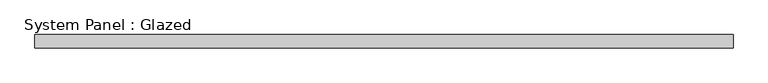
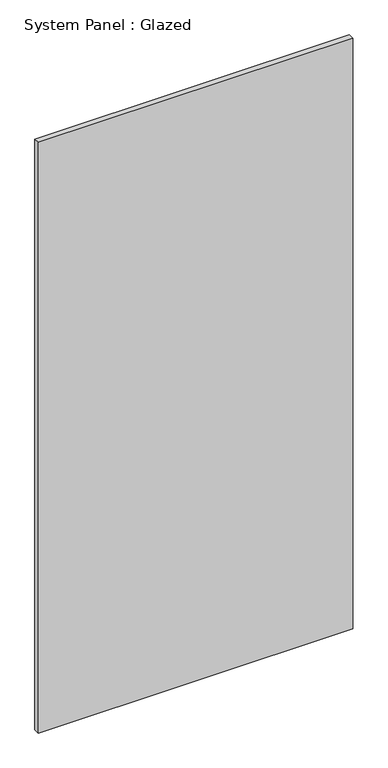
"""IFC4 building model written with IfcOpenShell, lengths in millimetres: plate geometry, System Panel : Glazed."""

from ifc_helpers import new_model, si_unit, origin, origin_with_axes, place, context, project, spatial, polyline, outline, extrude, source, transform, mapped, element, save


def system_panel_glazed_8e2f599f(model_context):
    return source(origin(), model_context, "Body", "SweptSolid", [
        extrude(outline(polyline([(666.75, 19.05), (-666.75, 19.05), (-666.75, 44.45), (666.75, 44.45), (666.75, 19.05)])), origin_with_axes(), (0.0, 0.0, 1.0), 2647.95),
    ])


if __name__ == "__main__":
    model = new_model("IFC4")
    model_context = context("Model", 3, world=origin())
    ifc_project = project(units=[si_unit("LENGTHUNIT", "METRE", prefix="MILLI")], contexts=[model_context])
    site = spatial("IfcSite", under=ifc_project)
    building = spatial("IfcBuilding", under=site)
    placement = place(None, origin())
    system_panel_glazed_shape = system_panel_glazed_8e2f599f(model_context)
    element("IfcPlate", 1, ObjectType="System Panel : Glazed", at=placement, inside=building, context=model_context, shape_type="MappedRepresentation", body=[
        mapped(system_panel_glazed_shape, transform((0.0, 0.0, 0.0), x_axis=(1.0, 0.0, 0.0), y_axis=(0.0, 1.0, 0.0), z_axis=(0.0, 0.0, 1.0))),
    ])
    save(model, "model.ifc")

# Revit data of these elements
# Type "System Panel : Glazed"
#   Construction Type Id = "GSP4R"
#   Analytic Construction = "1/8 in Pilkington single glazing"
#   Visual Light Transmittance = 0.9
#   Solar Heat Gain Coefficient = 0.86
#   Heat Transfer Coefficient (U) = 1.18115 BTU/(h·ft²·°F)
# Element 1 (IfcPlate, "System Panel : Glazed")
#   Materials on its faces: "Glass"
# Materials
#   "Glass": class "Glass", colour RGB 0 128 192, transparency 0.75, Description = "Soda Lime Glass", Cost = 0
